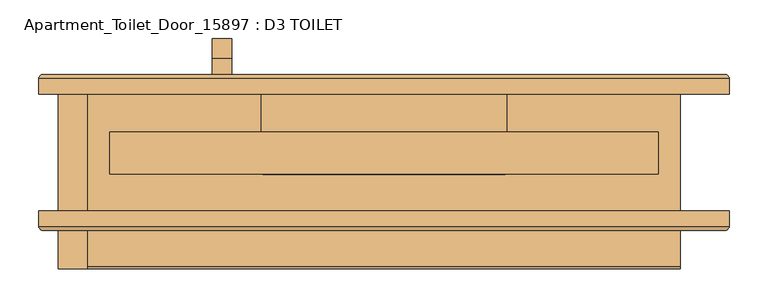
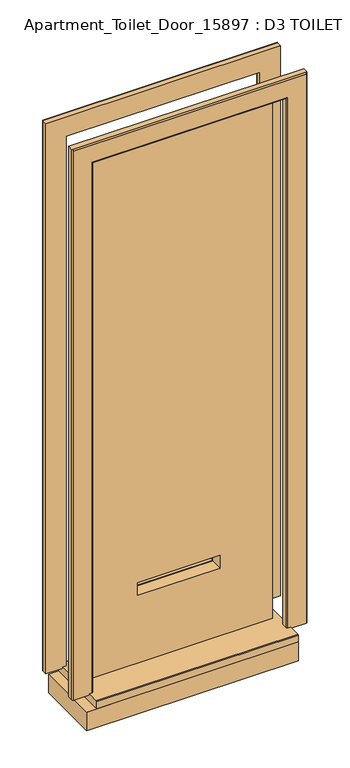
"""IFC4 building model written with IfcOpenShell, lengths in millimetres: door geometry, Apartment_Toilet_Door_15897 : D3 TOILET."""

from ifc_helpers import new_model, si_unit, frame, origin, place, context, project, spatial, polyline, circle_curve, ellipse_curve, outline, extrude, faceted_brep, source, transform, mapped, element, save
from ifc_brep_helpers import plane_surface, cylinder_surface, advanced_brep


def apartment_toilet_door_15897_d3_toilet_d7560075(model_context):
    return source(origin(), model_context, "Body", "SolidModel", [
        extrude(outline(polyline([(1241.0, -221.0), (1053.0132974, -221.0), (860.0, -221.0), (860.0, -196.0), (1050.7445158, -196.0), (1241.0, -196.0), (1241.0, -221.0)])), frame((0.0, 146.0, 0.0), z_axis=(0.0, 1.0, 0.0), x_axis=(0.0, 0.0, 1.0)), (0.0, 0.0, 1.0), 25.0),
        extrude(outline(polyline([(-196.0, 146.0), (-196.0, 100.0), (-221.0, 100.0), (-221.0, 146.0), (-196.0, 146.0)])), frame((0.0, 0.0, 1188.0), z_axis=(0.0, 0.0, 1.0), x_axis=(1.0, 0.0, 0.0)), (0.0, 0.0, 1.0), 25.0),
        extrude(outline(polyline([(-196.0, 146.0), (-196.0, 100.0), (-221.0, 100.0), (-221.0, 146.0), (-196.0, 146.0)])), frame((0.0, 0.0, 888.0), z_axis=(0.0, 0.0, 1.0), x_axis=(1.0, 0.0, 0.0)), (0.0, 0.0, 1.0), 25.0),
        extrude(outline(polyline([(-156.0, 46.0), (-156.0, 42.0), (-251.0, 42.0), (-251.0, 46.0), (-156.0, 46.0)])), frame((0.0, 0.0, 825.0), z_axis=(0.0, 0.0, 1.0), x_axis=(1.0, 0.0, 0.0)), (0.0, 0.0, 1.0), 451.0),
        extrude(outline(polyline([(2105.6000374, 353.0000374), (2105.6000374, -353.0000374), (5.0, -353.0000374), (5.0, 353.0000374), (2105.6000374, 353.0000374)]), holes=[polyline([(325.0, 156.0), (275.0, 156.0), (275.0, -156.0), (325.0, -156.0), (325.0, 156.0)])]), frame((0.0, -3.2, 0.0), z_axis=(0.0, 1.0, 0.0), x_axis=(0.0, 0.0, 1.0)), (0.0, 0.0, 1.0), 54.0),
        advanced_brep(
        [(-370.9983436, 125.0, 0.0), (-366.0, 120.0016564, 0.0), (-366.0, 100.0, 0.0), (-443.9993919, 100.0, 0.0), (-443.9993919, 119.9992678, 0.0), (-438.9986597, 125.0, 0.0), (-370.9983436, 125.0, 2123.5983436), (-366.0, 120.0016564, 2118.6), (-366.0, 100.0, 2118.6), (366.0, 100.0, 2118.6), (366.0, 100.0, 0.0), (443.9993919, 100.0, 0.0), (443.9993919, 100.0, 2196.5993919), (-443.9993919, 100.0, 2196.5993919), (-443.9993919, 119.9992678, 2196.5993919), (-438.9986597, 125.0, 2191.5986597), (438.9986597, 125.0, 2191.5986597), (438.9986597, 125.0, 0.0), (370.9983436, 125.0, 0.0), (370.9983436, 125.0, 2123.5983436), (366.0, 120.0016564, 2118.6), (366.0, 120.0016564, 0.0), (443.9993919, 119.9992678, 0.0), (443.9993919, 119.9992678, 2196.5993919)],
        [
            (0, 1, circle_curve(frame((-370.9983436, 120.0016564, 0.0), z_axis=(0.0, 0.0, -1.0), x_axis=(-1.0, 0.0, 0.0)), 4.9983436)),
            (1, 2),
            (2, 3),
            (3, 4),
            (4, 5, circle_curve(frame((-438.9986597, 119.9992678, 0.0), z_axis=(0.0, 0.0, -1.0), x_axis=(-1.0, 0.0, 0.0)), 5.0007322)),
            (5, 0),
            (0, 6),
            (6, 7, ellipse_curve(frame((-370.9983436, 120.0016564, 2123.5983436), z_axis=(-0.7071067811865475, 0.0, -0.7071067811865475), x_axis=(0.7071067811865474, 0.0, -0.7071067811865476)), 7.0687253, 4.9983436)),
            (7, 1),
            (7, 8),
            (8, 2),
            (8, 9),
            (9, 10),
            (10, 11),
            (11, 12),
            (12, 13),
            (13, 3),
            (13, 14),
            (14, 4),
            (14, 15, ellipse_curve(frame((-438.9986597, 119.9992678, 2191.5986597), z_axis=(-0.7071067811865475, 0.0, -0.7071067811865475), x_axis=(0.7071067811865474, 0.0, -0.7071067811865476)), 7.0721032, 5.0007322)),
            (15, 5),
            (15, 16),
            (16, 17),
            (17, 18),
            (18, 19),
            (19, 6),
            (9, 20),
            (20, 21),
            (21, 10),
            (17, 22, circle_curve(frame((438.9986597, 119.9992678, 0.0), z_axis=(0.0, 0.0, -1.0), x_axis=(1.0, 0.0, 0.0)), 5.0007322)),
            (22, 11),
            (21, 18, circle_curve(frame((370.9983436, 120.0016564, 0.0), z_axis=(0.0, 0.0, -1.0), x_axis=(1.0, 0.0, 0.0)), 4.9983436)),
            (23, 12),
            (22, 23),
            (16, 23, ellipse_curve(frame((438.9986597, 119.9992678, 2191.5986597), z_axis=(0.7071067811865475, 0.0, -0.7071067811865475), x_axis=(0.7071067811865474, 0.0, 0.7071067811865476)), 7.0721032, 5.0007322)),
            (20, 19, ellipse_curve(frame((370.9983436, 120.0016564, 2123.5983436), z_axis=(0.7071067811865475, 0.0, -0.7071067811865475), x_axis=(0.7071067811865474, 0.0, 0.7071067811865476)), 7.0687253, 4.9983436)),
            (20, 7),
            (23, 14),
        ],
        [
            plane_surface(frame((-381.0, -125.0, 0.0), z_axis=(0.0, 0.0, -1.0), x_axis=(0.0, -1.0, 0.0))),
            cylinder_surface(frame((-370.9983436, 120.0016564, 0.0), z_axis=(0.0, 0.0, -1.0), x_axis=(-1.0, 0.0, 0.0)), 4.9983436),
            plane_surface(frame((-366.0, 120.0016564, 0.0), z_axis=(1.0, 0.0, 0.0), x_axis=(0.0, 0.0, 1.0))),
            plane_surface(frame((-366.0, 100.0, 0.0), z_axis=(0.0, -1.0, 0.0), x_axis=(0.0, 0.0, 1.0))),
            plane_surface(frame((-443.9993919, 100.0, 0.0), z_axis=(-1.0, 0.0, 0.0), x_axis=(0.0, 0.0, 1.0))),
            cylinder_surface(frame((-438.9986597, 119.9992678, 0.0), z_axis=(0.0, 0.0, -1.0), x_axis=(-1.0, 0.0, 0.0)), 5.0007322),
            plane_surface(frame((-438.9986597, 125.0, 0.0), z_axis=(0.0, 1.0, 0.0), x_axis=(0.0, 0.0, 1.0))),
            plane_surface(frame((366.0, 120.0016564, 2118.6), z_axis=(-1.0, 0.0, 0.0), x_axis=(0.0, 0.0, -1.0))),
            plane_surface(frame((381.0, -125.0, 0.0), z_axis=(0.0, 0.0, -1.0), x_axis=(0.0, -1.0, 0.0))),
            plane_surface(frame((443.9993919, 100.0, 2196.5993919), z_axis=(1.0, 0.0, 0.0), x_axis=(0.0, 0.0, -1.0))),
            cylinder_surface(frame((438.9986597, 119.9992678, 2133.6), z_axis=(0.0, 0.0, 1.0), x_axis=(1.0, 0.0, 0.0)), 5.0007322),
            cylinder_surface(frame((370.9983436, 120.0016564, 2133.6), z_axis=(0.0, 0.0, 1.0), x_axis=(1.0, 0.0, 0.0)), 4.9983436),
            cylinder_surface(frame((-381.0, 120.0016564, 2123.5983436), z_axis=(-1.0, 0.0, 0.0), x_axis=(0.0, 0.0, 1.0)), 4.9983436),
            plane_surface(frame((-366.0, 120.0016564, 2118.6), z_axis=(0.0, 0.0, -1.0), x_axis=(1.0, 0.0, 0.0))),
            plane_surface(frame((-443.9993919, 100.0, 2196.5993919), z_axis=(0.0, 0.0, 1.0), x_axis=(1.0, 0.0, 0.0))),
            cylinder_surface(frame((-381.0, 119.9992678, 2191.5986597), z_axis=(-1.0, 0.0, 0.0), x_axis=(0.0, 0.0, 1.0)), 5.0007322),
        ],
        [
            (0, [[1, 2, 3, 4, 5, 6]]),
            (1, [[-1, 7, 8, 9]]),
            (2, [[-2, -9, 10, 11]]),
            (3, [[-3, -11, 12, 13, 14, 15, 16, 17]]),
            (4, [[-4, -17, 18, 19]]),
            (5, [[-5, -19, 20, 21]]),
            (6, [[-6, -21, 22, 23, 24, 25, 26, -7]]),
            (7, [[27, 28, 29, -13]]),
            (8, [[-24, 30, 31, -14, -29, 32]]),
            (9, [[33, -15, -31, 34]]),
            (10, [[35, -34, -30, -23]]),
            (11, [[36, -25, -32, -28]]),
            (12, [[-8, -26, -36, 37]]),
            (13, [[-10, -37, -27, -12]]),
            (14, [[-18, -16, -33, 38]]),
            (15, [[-20, -38, -35, -22]]),
        ],
    ),
        advanced_brep(
        [(-370.9983436, -75.8, 0.0), (-438.9986597, -75.8, 0.0), (-443.9993919, -70.7992678, 0.0), (-443.9993919, -50.8, 0.0), (-366.0, -50.8, 0.0), (-366.0, -70.8016564, 0.0), (-370.9983436, -75.8, 2123.5983436), (370.9983436, -75.8, 2123.5983436), (370.9983436, -75.8, 0.0), (438.9986597, -75.8, 0.0), (438.9986597, -75.8, 2191.5986597), (-438.9986597, -75.8, 2191.5986597), (-443.9993919, -70.7992678, 2196.5993919), (-443.9993919, -50.8, 2196.5993919), (443.9993919, -50.8, 2196.5993919), (443.9993919, -50.8, 0.0), (366.0, -50.8, 0.0), (366.0, -50.8, 2118.6), (-366.0, -50.8, 2118.6), (-366.0, -70.8016564, 2118.6), (443.9993919, -70.7992678, 2196.5993919), (443.9993919, -70.7992678, 0.0), (366.0, -70.8016564, 0.0), (366.0, -70.8016564, 2118.6)],
        [
            (0, 1),
            (1, 2, circle_curve(frame((-438.9986597, -70.7992678, 0.0), z_axis=(0.0, 0.0, -1.0), x_axis=(1.0, 0.0, 0.0)), 5.0007322)),
            (2, 3),
            (3, 4),
            (4, 5),
            (5, 0, circle_curve(frame((-370.9983436, -70.8016564, 0.0), z_axis=(0.0, 0.0, -1.0), x_axis=(1.0, 0.0, 0.0)), 4.9983436)),
            (0, 6),
            (6, 7),
            (7, 8),
            (8, 9),
            (9, 10),
            (10, 11),
            (11, 1),
            (11, 12, ellipse_curve(frame((-438.9986597, -70.7992678, 2191.5986597), z_axis=(-0.7071067811865475, 0.0, -0.7071067811865475), x_axis=(0.7071067811865474, 0.0, -0.7071067811865476)), 7.0721032, 5.0007322)),
            (12, 2),
            (12, 13),
            (13, 3),
            (13, 14),
            (14, 15),
            (15, 16),
            (16, 17),
            (17, 18),
            (18, 4),
            (18, 19),
            (19, 5),
            (19, 6, ellipse_curve(frame((-370.9983436, -70.8016564, 2123.5983436), z_axis=(-0.7071067811865475, 0.0, -0.7071067811865475), x_axis=(0.7071067811865474, 0.0, -0.7071067811865476)), 7.0687253, 4.9983436)),
            (14, 20),
            (20, 21),
            (21, 15),
            (8, 22, circle_curve(frame((370.9983436, -70.8016564, 0.0), z_axis=(0.0, 0.0, -1.0), x_axis=(-1.0, 0.0, 0.0)), 4.9983436)),
            (22, 16),
            (21, 9, circle_curve(frame((438.9986597, -70.7992678, 0.0), z_axis=(0.0, 0.0, -1.0), x_axis=(-1.0, 0.0, 0.0)), 5.0007322)),
            (23, 17),
            (22, 23),
            (7, 23, ellipse_curve(frame((370.9983436, -70.8016564, 2123.5983436), z_axis=(0.7071067811865475, 0.0, -0.7071067811865475), x_axis=(0.7071067811865474, 0.0, 0.7071067811865476)), 7.0687253, 4.9983436)),
            (20, 10, ellipse_curve(frame((438.9986597, -70.7992678, 2191.5986597), z_axis=(0.7071067811865475, 0.0, -0.7071067811865475), x_axis=(0.7071067811865474, 0.0, 0.7071067811865476)), 7.0721032, 5.0007322)),
            (19, 23),
            (12, 20),
        ],
        [
            plane_surface(frame((-381.0, 125.0, 0.0), z_axis=(0.0, 0.0, -1.0), x_axis=(0.0, 1.0, 0.0))),
            plane_surface(frame((-370.9983436, -75.8, 0.0), z_axis=(0.0, -1.0, 0.0), x_axis=(0.0, 0.0, 1.0))),
            cylinder_surface(frame((-438.9986597, -70.7992678, 0.0), z_axis=(0.0, 0.0, -1.0), x_axis=(1.0, 0.0, 0.0)), 5.0007322),
            plane_surface(frame((-443.9993919, -70.7992678, 0.0), z_axis=(-1.0, 0.0, 0.0), x_axis=(0.0, 0.0, 1.0))),
            plane_surface(frame((-443.9993919, -50.8, 0.0), z_axis=(0.0, 1.0, 0.0), x_axis=(0.0, 0.0, 1.0))),
            plane_surface(frame((-366.0, -50.8, 0.0), z_axis=(1.0, 0.0, 0.0), x_axis=(0.0, 0.0, 1.0))),
            cylinder_surface(frame((-370.9983436, -70.8016564, 0.0), z_axis=(0.0, 0.0, -1.0), x_axis=(1.0, 0.0, 0.0)), 4.9983436),
            plane_surface(frame((443.9993919, -70.7992678, 2196.5993919), z_axis=(1.0, 0.0, 0.0), x_axis=(0.0, 0.0, -1.0))),
            plane_surface(frame((381.0, 125.0, 0.0), z_axis=(0.0, 0.0, -1.0), x_axis=(0.0, 1.0, 0.0))),
            plane_surface(frame((366.0, -50.8, 2118.6), z_axis=(-1.0, 0.0, 0.0), x_axis=(0.0, 0.0, -1.0))),
            cylinder_surface(frame((370.9983436, -70.8016564, 2133.6), z_axis=(0.0, 0.0, 1.0), x_axis=(-1.0, 0.0, 0.0)), 4.9983436),
            cylinder_surface(frame((438.9986597, -70.7992678, 2133.6), z_axis=(0.0, 0.0, 1.0), x_axis=(-1.0, 0.0, 0.0)), 5.0007322),
            cylinder_surface(frame((-381.0, -70.8016564, 2123.5983436), z_axis=(-1.0, 0.0, 0.0), x_axis=(0.0, 0.0, -1.0)), 4.9983436),
            plane_surface(frame((-366.0, -50.8, 2118.6), z_axis=(0.0, 0.0, -1.0), x_axis=(1.0, 0.0, 0.0))),
            plane_surface(frame((-443.9993919, -70.7992678, 2196.5993919), z_axis=(0.0, 0.0, 1.0), x_axis=(1.0, 0.0, 0.0))),
            cylinder_surface(frame((-381.0, -70.7992678, 2191.5986597), z_axis=(-1.0, 0.0, 0.0), x_axis=(0.0, 0.0, -1.0)), 5.0007322),
        ],
        [
            (0, [[1, 2, 3, 4, 5, 6]]),
            (1, [[-1, 7, 8, 9, 10, 11, 12, 13]]),
            (2, [[-2, -13, 14, 15]]),
            (3, [[-3, -15, 16, 17]]),
            (4, [[-4, -17, 18, 19, 20, 21, 22, 23]]),
            (5, [[-5, -23, 24, 25]]),
            (6, [[-6, -25, 26, -7]]),
            (7, [[27, 28, 29, -19]]),
            (8, [[30, 31, -20, -29, 32, -10]]),
            (9, [[33, -21, -31, 34]]),
            (10, [[35, -34, -30, -9]]),
            (11, [[36, -11, -32, -28]]),
            (12, [[-26, 37, -35, -8]]),
            (13, [[-24, -22, -33, -37]]),
            (14, [[-16, 38, -27, -18]]),
            (15, [[-14, -12, -36, -38]]),
        ],
    ),
        extrude(outline(polyline([(-122.5, 5.0), (122.5, 5.0), (125.0, 2.5), (125.0, -25.0), (-125.0, -25.0), (-125.0, 2.5), (-122.5, 5.0)])), frame((-381.0, 0.0, 0.0), z_axis=(1.0, 0.0, 0.0), x_axis=(0.0, 1.0, 0.0)), (0.0, 0.0, 1.0), 762.0),
        extrude(outline(polyline([(-419.0, -125.0), (-419.0, 125.0), (381.0, 125.0), (381.0, -125.0), (-419.0, -125.0)])), frame((0.0, 0.0, -100.0), z_axis=(0.0, 0.0, 1.0), x_axis=(1.0, 0.0, 0.0)), (0.0, 0.0, 1.0), 75.0),
        faceted_brep([(168.0, 46.0, 265.0), (168.0, 44.0, 265.0), (-168.0, 44.0, 265.0), (-168.0, 46.0, 265.0), (158.0, 100.0, 275.0), (158.0, 46.0, 275.0), (-158.0, 46.0, 275.0), (-158.0, 100.0, 275.0), (168.0, 102.0, 265.0), (168.0, 100.0, 265.0), (-168.0, 100.0, 265.0), (-168.0, 102.0, 265.0), (155.0, 44.0, 278.0), (155.0, 102.0, 278.0), (-155.0, 102.0, 278.0), (-155.0, 44.0, 278.0), (-168.0, 46.0, 335.0), (-168.0, 44.0, 335.0), (168.0, 44.0, 335.0), (168.0, 46.0, 335.0), (-158.0, 100.0, 325.0), (-158.0, 46.0, 325.0), (158.0, 46.0, 325.0), (158.0, 100.0, 325.0), (-168.0, 102.0, 335.0), (-168.0, 100.0, 335.0), (168.0, 100.0, 335.0), (168.0, 102.0, 335.0), (-155.0, 44.0, 322.0), (-155.0, 102.0, 322.0), (155.0, 102.0, 322.0), (155.0, 44.0, 322.0)], [[[0, 1, 2, 3]], [[4, 5, 6, 7]], [[8, 9, 10, 11]], [[12, 13, 14, 15]], [[16, 17, 18, 19]], [[20, 21, 22, 23]], [[24, 25, 26, 27]], [[28, 29, 30, 31]], [[19, 18, 1, 0]], [[23, 22, 5, 4]], [[27, 26, 9, 8]], [[31, 30, 13, 12]], [[17, 2, 1, 18], [28, 31, 12, 15]], [[3, 2, 17, 16]], [[16, 19, 0, 3], [21, 6, 5, 22]], [[7, 6, 21, 20]], [[25, 10, 9, 26], [20, 23, 4, 7]], [[11, 10, 25, 24]], [[24, 27, 8, 11], [29, 14, 13, 30]], [[15, 14, 29, 28]]]),
    ])


if __name__ == "__main__":
    model = new_model("IFC4")
    model_context = context("Model", 3, world=origin())
    ifc_project = project(units=[si_unit("LENGTHUNIT", "METRE", prefix="MILLI")], contexts=[model_context])
    site = spatial("IfcSite", under=ifc_project)
    building = spatial("IfcBuilding", under=site)
    placement = place(None, origin())
    apartment_toilet_door_15897_d3_toilet_shape = apartment_toilet_door_15897_d3_toilet_d7560075(model_context)
    element("IfcDoor", 1, ObjectType="Apartment_Toilet_Door_15897 : D3 TOILET", at=placement, inside=building, context=model_context, shape_type="MappedRepresentation", body=[
        mapped(apartment_toilet_door_15897_d3_toilet_shape, transform((0.0, 0.0, 0.0), x_axis=(1.0, 0.0, 0.0), y_axis=(0.0, 1.0, 0.0), z_axis=(0.0, 0.0, 1.0))),
    ])
    save(model, "model.ifc")

# Revit data of these elements
# Type "Apartment_Toilet_Door_15897 : D3 TOILET"
#   Type Mark = "15"
#   Panel Type = ""
#   Location [instance default] = ""
#   Door Type = "Semi Solid Flushed Wooden Door Laminated on Boths Sides- Bathroom / Laundry"
#   Construction Type Id = "DOOR"
#   Analytic Construction = "Wooden"
#   Threshold Depth = 0' - 1.1811"
#   Thickness = 0' - 2.12598"
#   Thermal Resistance (R) = 2.58758 (h·ft²·°F)/BTU
#   Heat Transfer Coefficient (U) = 0.386456 BTU/(h·ft²·°F)
#   Height = 7' - 0"
#   Trim Projection Ext = 0' - 0.98425"
#   Trim Projection Int = 0' - 0.98425"
#   Width = 2' - 6"
#   Define Thermal Properties by = 1
#   Threshold Material = BEL-Threshold material-Marble
#   Visual Light Transmittance = 0
#   Solar Heat Gain Coefficient = 0
#   Function = (empty or 0)
#   Wall Closure = (empty or 0)
# Element 1 (IfcDoor, "Apartment_Toilet_Door_15897 : D3 TOILET")
#   Materials on its faces: "Default", "Metal - IR - Satin Chrome", "BEL-Threshold material-Marble", "BEL-Threshold material-Mortar"
# Materials
#   "BEL-Threshold material-Marble": colour RGB 197 197 199, transparency 0, Cost = 0
#   "Default": colour RGB 127 127 127, transparency 0, Cost = 0
#   "Metal - IR - Satin Chrome": colour RGB 244 244 244, transparency 0, Cost = 0
#   "BEL-Threshold material-Mortar": colour RGB 141 151 158, transparency 0, Cost = 0
